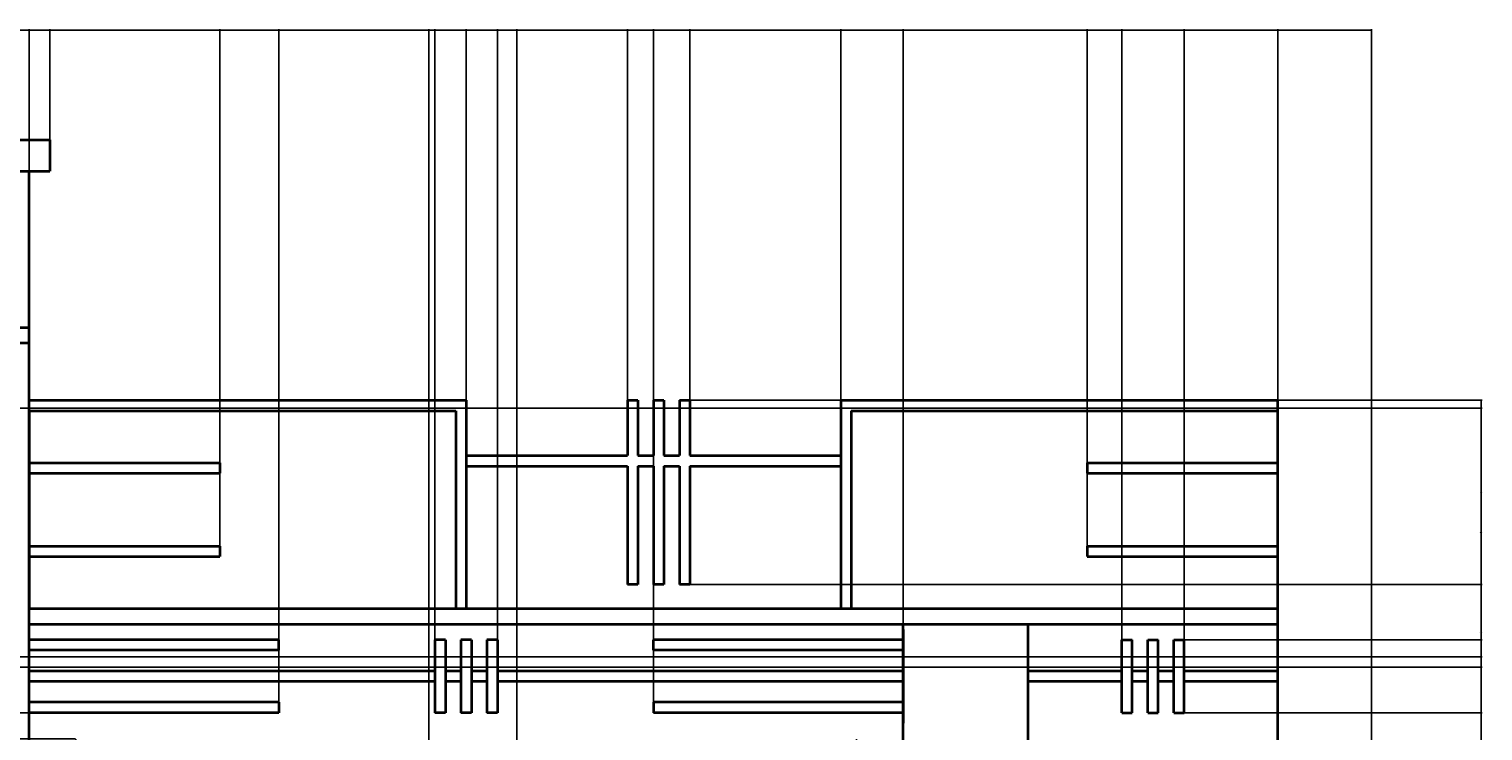
# Model space of a CAD drawing. Units: inches. Extents: x 2148 to 2587, y 1015 to 1466.
# Tile 7 of 7: x 2307 to 2586, y 1331 to 1466. Entities that reach past the tile are written whole.
import ezdxf

# ---------------------------------------------------------------- set-up
doc = ezdxf.new("R2010")
doc.units = ezdxf.units.IN
doc.layers.add('A-ANNO-DIMS', color=2, linetype='Continuous', lineweight=18)
doc.layers.add('A-ELEV', color=7, linetype='Continuous', lineweight=35)
doc.styles.get("Standard").update_dxf_attribs({"font": 'arial.ttf'})
doc.dimstyles.get("Standard").update_dxf_attribs({"dimtxt": 0.18, "dimasz": 0.18, "dimexe": 0.18, "dimexo": 0.0625, "dimgap": 0.09, "dimtad": 0, "dimtih": 1, "dimtoh": 1, "dimdec": 4, "dimzin": 0, "dimdsep": 46, "dimtxsty": 'Standard', "dimcen": 0.09, "dimadec": 0, "dimazin": 0, "dimtfac": 1, "dimtdec": 4, "dimtofl": 0, "dimtmove": 0, "dimatfit": 3, "dimfxl": 1, "dimtolj": 1, "dimtzin": 0, "dimarcsym": 0})

# ---------------------------------------------------------------- blocks, each defined once
blk = doc.blocks.new('*D8')
at = {"layer": 'A-ANNO-DIMS', "color": 0, "lineweight": -2, "transparency": 16777216}
for p, q in [((2183.03, 1444.81), (2183.03, 1466.02)), ((2183.21, 1465.84), (2246.75, 1465.84)), ((2310.85, 1465.84), (2247.31, 1465.84)), ((2311.03, 1444.81), (2311.03, 1466.02))]:
    blk.add_line(p, q, dxfattribs=at)
at = {"layer": 'A-ANNO-DIMS', "color": 0, "transparency": 16777216}
for points in [[(2183.21, 1465.87), (2183.21, 1465.81), (2183.03, 1465.84)], [(2310.85, 1465.87), (2310.85, 1465.81), (2311.03, 1465.84)]]:
    blk.add_solid(points, dxfattribs=at)
at = {"layer": 'Defpoints', "color": 0, "transparency": 16777216}
for p in [(2311.03, 1465.84), (2183.03, 1444.74), (2311.03, 1444.74)]:
    blk.add_point(p, dxfattribs=at)
at = {"layer": 'A-ANNO-DIMS', "color": 0, "transparency": 16777216, "insert": (2247.03, 1465.84), "char_height": 0.18, "attachment_point": 5}
blk.add_mtext('\\A1;128', dxfattribs=at)
blk = doc.blocks.new('*D9')
at = {"layer": 'A-ANNO-DIMS', "color": 0, "lineweight": -2, "transparency": 16777216}
for p, q in [((2311.03, 1444.81), (2311.03, 1466.02)), ((2311.21, 1465.84), (2437.74, 1465.84)), ((2564.85, 1465.84), (2438.32, 1465.84)), ((2565.03, 1305.54), (2565.03, 1466.02))]:
    blk.add_line(p, q, dxfattribs=at)
at = {"layer": 'A-ANNO-DIMS', "color": 0, "transparency": 16777216}
for points in [[(2311.21, 1465.87), (2311.21, 1465.81), (2311.03, 1465.84)], [(2564.85, 1465.87), (2564.85, 1465.81), (2565.03, 1465.84)]]:
    blk.add_solid(points, dxfattribs=at)
at = {"layer": 'Defpoints', "color": 0, "transparency": 16777216}
for p in [(2565.03, 1465.84), (2311.03, 1444.74), (2565.03, 1305.47)]:
    blk.add_point(p, dxfattribs=at)
at = {"layer": 'A-ANNO-DIMS', "color": 0, "transparency": 16777216, "insert": (2438.03, 1465.84), "char_height": 0.18, "attachment_point": 5}
blk.add_mtext('\\A1;254', dxfattribs=at)
blk = doc.blocks.new('*D32')
at = {"layer": 'A-ANNO-DIMS', "color": 0, "lineweight": -2, "transparency": 16777216}
for p, q in [((2547.1, 1394.74), (2586.31, 1394.74)), ((2586.13, 1394.56), (2586.13, 1350.29)), ((2586.13, 1305.65), (2586.13, 1349.93)), ((2565.1, 1305.47), (2586.31, 1305.47))]:
    blk.add_line(p, q, dxfattribs=at)
at = {"layer": 'A-ANNO-DIMS', "color": 0, "transparency": 16777216}
for points in [[(2586.1, 1394.56), (2586.16, 1394.56), (2586.13, 1394.74)], [(2586.1, 1305.65), (2586.16, 1305.65), (2586.13, 1305.47)]]:
    blk.add_solid(points, dxfattribs=at)
at = {"layer": 'Defpoints', "color": 0, "transparency": 16777216}
for p in [(2547.03, 1394.74), (2586.13, 1394.74), (2565.03, 1305.47)]:
    blk.add_point(p, dxfattribs=at)
at = {"layer": 'A-ANNO-DIMS', "color": 0, "transparency": 16777216, "insert": (2586.13, 1350.11), "char_height": 0.18, "attachment_point": 5}
blk.add_mtext('\\A1;89.27', dxfattribs=at)
blk = doc.blocks.new('*D33')
at = {"layer": 'A-ANNO-DIMS', "color": 0, "lineweight": -2, "transparency": 16777216}
for p, q in [((2307.03, 1394.81), (2307.03, 1466.02)), ((2307.21, 1465.84), (2324.89, 1465.84)), ((2343.5, 1465.84), (2325.82, 1465.84)), ((2343.68, 1366.81), (2343.68, 1466.02))]:
    blk.add_line(p, q, dxfattribs=at)
at = {"layer": 'A-ANNO-DIMS', "color": 0, "transparency": 16777216}
for points in [[(2307.21, 1465.87), (2307.21, 1465.81), (2307.03, 1465.84)], [(2343.5, 1465.87), (2343.5, 1465.81), (2343.68, 1465.84)]]:
    blk.add_solid(points, dxfattribs=at)
at = {"layer": 'Defpoints', "color": 0, "transparency": 16777216}
for p in [(2343.68, 1465.84), (2307.03, 1394.74), (2343.68, 1366.74)]:
    blk.add_point(p, dxfattribs=at)
at = {"layer": 'A-ANNO-DIMS', "color": 0, "transparency": 16777216, "insert": (2325.36, 1465.84), "char_height": 0.18, "attachment_point": 5}
blk.add_mtext('\\A1;36.645', dxfattribs=at)
blk = doc.blocks.new('*D34')
at = {"layer": 'A-ANNO-DIMS', "color": 0, "lineweight": -2, "transparency": 16777216}
for p, q in [((2343.68, 1366.81), (2343.68, 1466.02)), ((2343.86, 1465.84), (2348.9, 1465.84)), ((2354.85, 1465.84), (2349.81, 1465.84)), ((2355.03, 1334.81), (2355.03, 1466.02))]:
    blk.add_line(p, q, dxfattribs=at)
at = {"layer": 'A-ANNO-DIMS', "color": 0, "transparency": 16777216}
for points in [[(2343.86, 1465.87), (2343.86, 1465.81), (2343.68, 1465.84)], [(2354.85, 1465.87), (2354.85, 1465.81), (2355.03, 1465.84)]]:
    blk.add_solid(points, dxfattribs=at)
at = {"layer": 'Defpoints', "color": 0, "transparency": 16777216}
for p in [(2355.03, 1465.84), (2343.68, 1366.74), (2355.03, 1334.74)]:
    blk.add_point(p, dxfattribs=at)
at = {"layer": 'A-ANNO-DIMS', "color": 0, "transparency": 16777216, "insert": (2349.36, 1465.84), "char_height": 0.18, "attachment_point": 5}
blk.add_mtext('\\A1;11.355', dxfattribs=at)
blk = doc.blocks.new('*D35')
at = {"layer": 'A-ANNO-DIMS', "color": 0, "lineweight": -2, "transparency": 16777216}
for p, q in [((2355.03, 1334.81), (2355.03, 1466.02)), ((2355.21, 1465.84), (2369.82, 1465.84)), ((2384.85, 1465.84), (2370.25, 1465.84)), ((2385.03, 1334.81), (2385.03, 1466.02))]:
    blk.add_line(p, q, dxfattribs=at)
at = {"layer": 'A-ANNO-DIMS', "color": 0, "transparency": 16777216}
for points in [[(2355.21, 1465.87), (2355.21, 1465.81), (2355.03, 1465.84)], [(2384.85, 1465.87), (2384.85, 1465.81), (2385.03, 1465.84)]]:
    blk.add_solid(points, dxfattribs=at)
at = {"layer": 'Defpoints', "color": 0, "transparency": 16777216}
for p in [(2385.03, 1465.84), (2355.03, 1334.74), (2385.03, 1334.74)]:
    blk.add_point(p, dxfattribs=at)
at = {"layer": 'A-ANNO-DIMS', "color": 0, "transparency": 16777216, "insert": (2370.03, 1465.84), "char_height": 0.18, "attachment_point": 5}
blk.add_mtext('\\A1;30', dxfattribs=at)
blk = doc.blocks.new('*D36')
at = {"layer": 'A-ANNO-DIMS', "color": 0, "lineweight": -2, "transparency": 16777216}
for p, q in [((2385.03, 1334.81), (2385.03, 1466.02)), ((2385.21, 1465.84), (2387.88, 1465.84)), ((2390.85, 1465.84), (2388.18, 1465.84)), ((2391.03, 1394.81), (2391.03, 1466.02))]:
    blk.add_line(p, q, dxfattribs=at)
at = {"layer": 'A-ANNO-DIMS', "color": 0, "transparency": 16777216}
for points in [[(2385.21, 1465.87), (2385.21, 1465.81), (2385.03, 1465.84)], [(2390.85, 1465.87), (2390.85, 1465.81), (2391.03, 1465.84)]]:
    blk.add_solid(points, dxfattribs=at)
at = {"layer": 'Defpoints', "color": 0, "transparency": 16777216}
for p in [(2391.03, 1465.84), (2391.03, 1394.74), (2385.03, 1334.74)]:
    blk.add_point(p, dxfattribs=at)
at = {"layer": 'A-ANNO-DIMS', "color": 0, "transparency": 16777216, "insert": (2388.03, 1465.84), "char_height": 0.18, "attachment_point": 5}
blk.add_mtext('\\A1;6', dxfattribs=at)
blk = doc.blocks.new('*D37')
at = {"layer": 'A-ANNO-DIMS', "color": 0, "lineweight": -2, "transparency": 16777216}
for p, q in [((2391.03, 1394.81), (2391.03, 1466.02)), ((2391.21, 1465.84), (2393.88, 1465.84)), ((2396.85, 1465.84), (2394.18, 1465.84)), ((2397.03, 1334.81), (2397.03, 1466.02))]:
    blk.add_line(p, q, dxfattribs=at)
at = {"layer": 'A-ANNO-DIMS', "color": 0, "transparency": 16777216}
for points in [[(2391.21, 1465.87), (2391.21, 1465.81), (2391.03, 1465.84)], [(2396.85, 1465.87), (2396.85, 1465.81), (2397.03, 1465.84)]]:
    blk.add_solid(points, dxfattribs=at)
at = {"layer": 'Defpoints', "color": 0, "transparency": 16777216}
for p in [(2397.03, 1465.84), (2391.03, 1394.74), (2397.03, 1334.74)]:
    blk.add_point(p, dxfattribs=at)
at = {"layer": 'A-ANNO-DIMS', "color": 0, "transparency": 16777216, "insert": (2394.03, 1465.84), "char_height": 0.18, "attachment_point": 5}
blk.add_mtext('\\A1;6', dxfattribs=at)
blk = doc.blocks.new('*D38')
at = {"layer": 'A-ANNO-DIMS', "color": 0, "lineweight": -2, "transparency": 16777216}
for p, q in [((2397.03, 1334.81), (2397.03, 1466.02)), ((2397.21, 1465.84), (2409.31, 1465.84)), ((2421.85, 1465.84), (2409.76, 1465.84)), ((2422.03, 1394.81), (2422.03, 1466.02))]:
    blk.add_line(p, q, dxfattribs=at)
at = {"layer": 'A-ANNO-DIMS', "color": 0, "transparency": 16777216}
for points in [[(2397.21, 1465.87), (2397.21, 1465.81), (2397.03, 1465.84)], [(2421.85, 1465.87), (2421.85, 1465.81), (2422.03, 1465.84)]]:
    blk.add_solid(points, dxfattribs=at)
at = {"layer": 'Defpoints', "color": 0, "transparency": 16777216}
for p in [(2422.03, 1465.84), (2422.03, 1394.74), (2397.03, 1334.74)]:
    blk.add_point(p, dxfattribs=at)
at = {"layer": 'A-ANNO-DIMS', "color": 0, "transparency": 16777216, "insert": (2409.53, 1465.84), "char_height": 0.18, "attachment_point": 5}
blk.add_mtext('\\A1;25', dxfattribs=at)
blk = doc.blocks.new('*D39')
at = {"layer": 'A-ANNO-DIMS', "color": 0, "lineweight": -2, "transparency": 16777216}
for p, q in [((2422.03, 1394.81), (2422.03, 1466.02)), ((2422.21, 1465.84), (2424.38, 1465.84)), ((2426.85, 1465.84), (2424.68, 1465.84)), ((2427.03, 1334.81), (2427.03, 1466.02))]:
    blk.add_line(p, q, dxfattribs=at)
at = {"layer": 'A-ANNO-DIMS', "color": 0, "transparency": 16777216}
for points in [[(2422.21, 1465.87), (2422.21, 1465.81), (2422.03, 1465.84)], [(2426.85, 1465.87), (2426.85, 1465.81), (2427.03, 1465.84)]]:
    blk.add_solid(points, dxfattribs=at)
at = {"layer": 'Defpoints', "color": 0, "transparency": 16777216}
for p in [(2427.03, 1465.84), (2422.03, 1394.74), (2427.03, 1334.74)]:
    blk.add_point(p, dxfattribs=at)
at = {"layer": 'A-ANNO-DIMS', "color": 0, "transparency": 16777216, "insert": (2424.53, 1465.84), "char_height": 0.18, "attachment_point": 5}
blk.add_mtext('\\A1;5', dxfattribs=at)
blk = doc.blocks.new('*D40')
at = {"layer": 'A-ANNO-DIMS', "color": 0, "lineweight": -2, "transparency": 16777216}
for p, q in [((2427.03, 1334.81), (2427.03, 1466.02)), ((2427.21, 1465.84), (2430.39, 1465.84)), ((2433.85, 1465.84), (2430.68, 1465.84)), ((2434.03, 1394.81), (2434.03, 1466.02))]:
    blk.add_line(p, q, dxfattribs=at)
at = {"layer": 'A-ANNO-DIMS', "color": 0, "transparency": 16777216}
for points in [[(2427.21, 1465.87), (2427.21, 1465.81), (2427.03, 1465.84)], [(2433.85, 1465.87), (2433.85, 1465.81), (2434.03, 1465.84)]]:
    blk.add_solid(points, dxfattribs=at)
at = {"layer": 'Defpoints', "color": 0, "transparency": 16777216}
for p in [(2434.03, 1465.84), (2434.03, 1394.74), (2427.03, 1334.74)]:
    blk.add_point(p, dxfattribs=at)
at = {"layer": 'A-ANNO-DIMS', "color": 0, "transparency": 16777216, "insert": (2430.53, 1465.84), "char_height": 0.18, "attachment_point": 5}
blk.add_mtext('\\A1;7', dxfattribs=at)
blk = doc.blocks.new('*D41')
at = {"layer": 'A-ANNO-DIMS', "color": 0, "lineweight": -2, "transparency": 16777216}
for p, q in [((2434.03, 1394.81), (2434.03, 1466.02)), ((2434.21, 1465.84), (2448.31, 1465.84)), ((2462.85, 1465.84), (2448.75, 1465.84)), ((2463.03, 1394.81), (2463.03, 1466.02))]:
    blk.add_line(p, q, dxfattribs=at)
at = {"layer": 'A-ANNO-DIMS', "color": 0, "transparency": 16777216}
for points in [[(2434.21, 1465.87), (2434.21, 1465.81), (2434.03, 1465.84)], [(2462.85, 1465.87), (2462.85, 1465.81), (2463.03, 1465.84)]]:
    blk.add_solid(points, dxfattribs=at)
at = {"layer": 'Defpoints', "color": 0, "transparency": 16777216}
for p in [(2463.03, 1465.84), (2434.03, 1394.74), (2463.03, 1394.74)]:
    blk.add_point(p, dxfattribs=at)
at = {"layer": 'A-ANNO-DIMS', "color": 0, "transparency": 16777216, "insert": (2448.53, 1465.84), "char_height": 0.18, "attachment_point": 5}
blk.add_mtext('\\A1;29', dxfattribs=at)
blk = doc.blocks.new('*D42')
at = {"layer": 'A-ANNO-DIMS', "color": 0, "lineweight": -2, "transparency": 16777216}
for p, q in [((2463.03, 1394.81), (2463.03, 1466.02)), ((2463.21, 1465.84), (2468.82, 1465.84)), ((2474.85, 1465.84), (2469.24, 1465.84)), ((2475.03, 1351.81), (2475.03, 1466.02))]:
    blk.add_line(p, q, dxfattribs=at)
at = {"layer": 'A-ANNO-DIMS', "color": 0, "transparency": 16777216}
for points in [[(2463.21, 1465.87), (2463.21, 1465.81), (2463.03, 1465.84)], [(2474.85, 1465.87), (2474.85, 1465.81), (2475.03, 1465.84)]]:
    blk.add_solid(points, dxfattribs=at)
at = {"layer": 'Defpoints', "color": 0, "transparency": 16777216}
for p in [(2475.03, 1465.84), (2463.03, 1394.74), (2475.03, 1351.74)]:
    blk.add_point(p, dxfattribs=at)
at = {"layer": 'A-ANNO-DIMS', "color": 0, "transparency": 16777216, "insert": (2469.03, 1465.84), "char_height": 0.18, "attachment_point": 5}
blk.add_mtext('\\A1;12', dxfattribs=at)
blk = doc.blocks.new('*D43')
at = {"layer": 'A-ANNO-DIMS', "color": 0, "lineweight": -2, "transparency": 16777216}
for p, q in [((2475.03, 1351.81), (2475.03, 1466.02)), ((2475.21, 1465.84), (2492.25, 1465.84)), ((2510.21, 1465.84), (2493.18, 1465.84)), ((2510.39, 1366.81), (2510.39, 1466.02))]:
    blk.add_line(p, q, dxfattribs=at)
at = {"layer": 'A-ANNO-DIMS', "color": 0, "transparency": 16777216}
for points in [[(2475.21, 1465.87), (2475.21, 1465.81), (2475.03, 1465.84)], [(2510.21, 1465.87), (2510.21, 1465.81), (2510.39, 1465.84)]]:
    blk.add_solid(points, dxfattribs=at)
at = {"layer": 'Defpoints', "color": 0, "transparency": 16777216}
for p in [(2510.39, 1465.84), (2510.39, 1366.74), (2475.03, 1351.74)]:
    blk.add_point(p, dxfattribs=at)
at = {"layer": 'A-ANNO-DIMS', "color": 0, "transparency": 16777216, "insert": (2492.71, 1465.84), "char_height": 0.18, "attachment_point": 5}
blk.add_mtext('\\A1;35.355', dxfattribs=at)
blk = doc.blocks.new('*D44')
at = {"layer": 'A-ANNO-DIMS', "color": 0, "lineweight": -2, "transparency": 16777216}
for p, q in [((2510.39, 1366.81), (2510.39, 1466.02)), ((2510.57, 1465.84), (2513.32, 1465.84)), ((2516.85, 1465.84), (2514.11, 1465.84)), ((2517.03, 1334.81), (2517.03, 1466.02))]:
    blk.add_line(p, q, dxfattribs=at)
at = {"layer": 'A-ANNO-DIMS', "color": 0, "transparency": 16777216}
for points in [[(2510.57, 1465.87), (2510.57, 1465.81), (2510.39, 1465.84)], [(2516.85, 1465.87), (2516.85, 1465.81), (2517.03, 1465.84)]]:
    blk.add_solid(points, dxfattribs=at)
at = {"layer": 'Defpoints', "color": 0, "transparency": 16777216}
for p in [(2517.03, 1465.84), (2510.39, 1366.74), (2517.03, 1334.74)]:
    blk.add_point(p, dxfattribs=at)
at = {"layer": 'A-ANNO-DIMS', "color": 0, "transparency": 16777216, "insert": (2513.71, 1465.84), "char_height": 0.18, "attachment_point": 5}
blk.add_mtext('\\A1;6.645', dxfattribs=at)
blk = doc.blocks.new('*D45')
at = {"layer": 'A-ANNO-DIMS', "color": 0, "lineweight": -2, "transparency": 16777216}
for p, q in [((2517.03, 1334.81), (2517.03, 1466.02)), ((2517.21, 1465.84), (2522.82, 1465.84)), ((2528.85, 1465.84), (2523.24, 1465.84)), ((2529.03, 1334.81), (2529.03, 1466.02))]:
    blk.add_line(p, q, dxfattribs=at)
at = {"layer": 'A-ANNO-DIMS', "color": 0, "transparency": 16777216}
for points in [[(2517.21, 1465.87), (2517.21, 1465.81), (2517.03, 1465.84)], [(2528.85, 1465.87), (2528.85, 1465.81), (2529.03, 1465.84)]]:
    blk.add_solid(points, dxfattribs=at)
at = {"layer": 'Defpoints', "color": 0, "transparency": 16777216}
for p in [(2529.03, 1465.84), (2517.03, 1334.74), (2529.03, 1334.74)]:
    blk.add_point(p, dxfattribs=at)
at = {"layer": 'A-ANNO-DIMS', "color": 0, "transparency": 16777216, "insert": (2523.03, 1465.84), "char_height": 0.18, "attachment_point": 5}
blk.add_mtext('\\A1;12', dxfattribs=at)
blk = doc.blocks.new('*D46')
at = {"layer": 'A-ANNO-DIMS', "color": 0, "lineweight": -2, "transparency": 16777216}
for p, q in [((2529.03, 1334.81), (2529.03, 1466.02)), ((2529.21, 1465.84), (2537.82, 1465.84)), ((2546.85, 1465.84), (2538.24, 1465.84)), ((2547.03, 1394.81), (2547.03, 1466.02))]:
    blk.add_line(p, q, dxfattribs=at)
at = {"layer": 'A-ANNO-DIMS', "color": 0, "transparency": 16777216}
for points in [[(2529.21, 1465.87), (2529.21, 1465.81), (2529.03, 1465.84)], [(2546.85, 1465.87), (2546.85, 1465.81), (2547.03, 1465.84)]]:
    blk.add_solid(points, dxfattribs=at)
at = {"layer": 'Defpoints', "color": 0, "transparency": 16777216}
for p in [(2547.03, 1465.84), (2547.03, 1394.74), (2529.03, 1334.74)]:
    blk.add_point(p, dxfattribs=at)
at = {"layer": 'A-ANNO-DIMS', "color": 0, "transparency": 16777216, "insert": (2538.03, 1465.84), "char_height": 0.18, "attachment_point": 5}
blk.add_mtext('\\A1;18', dxfattribs=at)
blk = doc.blocks.new('*D47')
at = {"layer": 'A-ANNO-DIMS', "color": 0, "lineweight": -2, "transparency": 16777216}
for p, q in [((2307.03, 1334.68), (2307.03, 1015.46)), ((2316.03, 1329.68), (2316.03, 1015.46)), ((2307.21, 1015.64), (2311.39, 1015.64)), ((2315.85, 1015.64), (2311.68, 1015.64))]:
    blk.add_line(p, q, dxfattribs=at)
at = {"layer": 'A-ANNO-DIMS', "color": 0, "transparency": 16777216}
for points in [[(2307.21, 1015.67), (2307.21, 1015.61), (2307.03, 1015.64)], [(2315.85, 1015.67), (2315.85, 1015.61), (2316.03, 1015.64)]]:
    blk.add_solid(points, dxfattribs=at)
at = {"layer": 'Defpoints', "color": 0, "transparency": 16777216}
for p in [(2307.03, 1334.74), (2316.03, 1329.74), (2316.03, 1015.64)]:
    blk.add_point(p, dxfattribs=at)
at = {"layer": 'A-ANNO-DIMS', "color": 0, "transparency": 16777216, "insert": (2311.53, 1015.64), "char_height": 0.18, "attachment_point": 5}
blk.add_mtext('\\A1;9', dxfattribs=at)
blk = doc.blocks.new('*D53')
at = {"layer": 'A-ANNO-DIMS', "color": 0, "lineweight": -2, "transparency": 16777216}
for p, q in [((2475.03, 1351.68), (2475.03, 1015.46)), ((2466.03, 1329.68), (2466.03, 1015.46)), ((2466.21, 1015.64), (2470.39, 1015.64)), ((2474.85, 1015.64), (2470.68, 1015.64))]:
    blk.add_line(p, q, dxfattribs=at)
at = {"layer": 'A-ANNO-DIMS', "color": 0, "transparency": 16777216}
for points in [[(2466.21, 1015.67), (2466.21, 1015.61), (2466.03, 1015.64)], [(2474.85, 1015.67), (2474.85, 1015.61), (2475.03, 1015.64)]]:
    blk.add_solid(points, dxfattribs=at)
at = {"layer": 'Defpoints', "color": 0, "transparency": 16777216}
for p in [(2475.03, 1351.74), (2466.03, 1329.74), (2475.03, 1015.64)]:
    blk.add_point(p, dxfattribs=at)
at = {"layer": 'A-ANNO-DIMS', "color": 0, "transparency": 16777216, "insert": (2470.53, 1015.64), "char_height": 0.18, "attachment_point": 5}
blk.add_mtext('\\A1;9', dxfattribs=at)
blk = doc.blocks.new('*D54')
at = {"layer": 'A-ANNO-DIMS', "color": 0, "lineweight": -2, "transparency": 16777216}
for p, q in [((2475.03, 1351.68), (2475.03, 1015.46)), ((2499.03, 1329.68), (2499.03, 1015.46)), ((2475.21, 1015.64), (2486.81, 1015.64)), ((2498.85, 1015.64), (2487.25, 1015.64))]:
    blk.add_line(p, q, dxfattribs=at)
at = {"layer": 'A-ANNO-DIMS', "color": 0, "transparency": 16777216}
for points in [[(2475.21, 1015.67), (2475.21, 1015.61), (2475.03, 1015.64)], [(2498.85, 1015.67), (2498.85, 1015.61), (2499.03, 1015.64)]]:
    blk.add_solid(points, dxfattribs=at)
at = {"layer": 'Defpoints', "color": 0, "transparency": 16777216}
for p in [(2475.03, 1351.74), (2499.03, 1329.74), (2499.03, 1015.64)]:
    blk.add_point(p, dxfattribs=at)
at = {"layer": 'A-ANNO-DIMS', "color": 0, "transparency": 16777216, "insert": (2487.03, 1015.64), "char_height": 0.18, "attachment_point": 5}
blk.add_mtext('\\A1;24', dxfattribs=at)
blk = doc.blocks.new('*D63')
at = {"layer": 'A-ANNO-DIMS', "color": 0, "lineweight": -2, "transparency": 16777216}
for p, q in [((2306.97, 1334.74), (2147.75, 1334.74)), ((2147.93, 1334.56), (2147.93, 1332.42)), ((2147.93, 1329.92), (2147.93, 1332.06)), ((2315.97, 1329.74), (2147.75, 1329.74))]:
    blk.add_line(p, q, dxfattribs=at)
at = {"layer": 'A-ANNO-DIMS', "color": 0, "transparency": 16777216}
for points in [[(2147.9, 1334.56), (2147.96, 1334.56), (2147.93, 1334.74)], [(2147.9, 1329.92), (2147.96, 1329.92), (2147.93, 1329.74)]]:
    blk.add_solid(points, dxfattribs=at)
at = {"layer": 'Defpoints', "color": 0, "transparency": 16777216}
for p in [(2147.93, 1334.74), (2307.03, 1334.74), (2316.03, 1329.74)]:
    blk.add_point(p, dxfattribs=at)
at = {"layer": 'A-ANNO-DIMS', "color": 0, "transparency": 16777216, "insert": (2147.93, 1332.24), "char_height": 0.18, "attachment_point": 5}
blk.add_mtext('\\A1;5', dxfattribs=at)
blk = doc.blocks.new('*D71')
at = {"layer": 'A-ANNO-DIMS', "color": 0, "lineweight": -2, "transparency": 16777216}
for p, q in [((2529.1, 1348.74), (2586.31, 1348.74)), ((2586.13, 1348.56), (2586.13, 1341.92)), ((2586.13, 1334.92), (2586.13, 1341.56)), ((2529.1, 1334.74), (2586.31, 1334.74))]:
    blk.add_line(p, q, dxfattribs=at)
at = {"layer": 'A-ANNO-DIMS', "color": 0, "transparency": 16777216}
for points in [[(2586.1, 1348.56), (2586.16, 1348.56), (2586.13, 1348.74)], [(2586.1, 1334.92), (2586.16, 1334.92), (2586.13, 1334.74)]]:
    blk.add_solid(points, dxfattribs=at)
at = {"layer": 'Defpoints', "color": 0, "transparency": 16777216}
for p in [(2529.03, 1348.74), (2586.13, 1348.74), (2529.03, 1334.74)]:
    blk.add_point(p, dxfattribs=at)
at = {"layer": 'A-ANNO-DIMS', "color": 0, "transparency": 16777216, "insert": (2586.13, 1341.74), "char_height": 0.18, "attachment_point": 5}
blk.add_mtext('\\A1;14', dxfattribs=at)
blk = doc.blocks.new('*D72')
at = {"layer": 'A-ANNO-DIMS', "color": 0, "lineweight": -2, "transparency": 16777216}
for p, q in [((2434.1, 1394.74), (2586.31, 1394.74)), ((2586.13, 1394.56), (2586.13, 1377.24)), ((2586.13, 1359.56), (2586.13, 1376.88)), ((2434.1, 1359.38), (2586.31, 1359.38))]:
    blk.add_line(p, q, dxfattribs=at)
at = {"layer": 'A-ANNO-DIMS', "color": 0, "transparency": 16777216}
for points in [[(2586.1, 1394.56), (2586.16, 1394.56), (2586.13, 1394.74)], [(2586.1, 1359.56), (2586.16, 1359.56), (2586.13, 1359.38)]]:
    blk.add_solid(points, dxfattribs=at)
at = {"layer": 'Defpoints', "color": 0, "transparency": 16777216}
for p in [(2434.03, 1394.74), (2586.13, 1394.74), (2434.03, 1359.38)]:
    blk.add_point(p, dxfattribs=at)
at = {"layer": 'A-ANNO-DIMS', "color": 0, "transparency": 16777216, "insert": (2586.13, 1377.06), "char_height": 0.18, "attachment_point": 5}
blk.add_mtext('\\A1;35.37', dxfattribs=at)
blk = doc.blocks.new('*D95')
at = {"layer": 'A-ANNO-DIMS', "color": 0, "lineweight": -2, "transparency": 16777216}
for p, q in [((2260.35, 1343.49), (2586.31, 1343.49)), ((2586.13, 1343.31), (2586.13, 1295.67)), ((2586.13, 1247.67), (2586.13, 1295.31)), ((2260.35, 1247.49), (2586.31, 1247.49))]:
    blk.add_line(p, q, dxfattribs=at)
at = {"layer": 'A-ANNO-DIMS', "color": 0, "transparency": 16777216}
for points in [[(2586.1, 1343.31), (2586.16, 1343.31), (2586.13, 1343.49)], [(2586.1, 1247.67), (2586.16, 1247.67), (2586.13, 1247.49)]]:
    blk.add_solid(points, dxfattribs=at)
at = {"layer": 'Defpoints', "color": 0, "transparency": 16777216}
for p in [(2260.29, 1343.49), (2586.13, 1343.49), (2260.29, 1247.49)]:
    blk.add_point(p, dxfattribs=at)
at = {"layer": 'A-ANNO-DIMS', "color": 0, "transparency": 16777216, "insert": (2586.13, 1295.49), "char_height": 0.18, "attachment_point": 5}
blk.add_mtext('\\A1;96', dxfattribs=at)
blk = doc.blocks.new('*D96')
at = {"layer": 'A-ANNO-DIMS', "color": 0, "lineweight": -2, "transparency": 16777216}
for p, q in [((2260.35, 1345.49), (2586.31, 1345.49)), ((2586.13, 1345.31), (2586.13, 1344.67)), ((2586.13, 1343.67), (2586.13, 1344.31)), ((2260.35, 1343.49), (2586.31, 1343.49))]:
    blk.add_line(p, q, dxfattribs=at)
at = {"layer": 'A-ANNO-DIMS', "color": 0, "transparency": 16777216}
for points in [[(2586.1, 1345.31), (2586.16, 1345.31), (2586.13, 1345.49)], [(2586.1, 1343.67), (2586.16, 1343.67), (2586.13, 1343.49)]]:
    blk.add_solid(points, dxfattribs=at)
at = {"layer": 'Defpoints', "color": 0, "transparency": 16777216}
for p in [(2260.29, 1345.49), (2586.13, 1345.49), (2260.29, 1343.49)]:
    blk.add_point(p, dxfattribs=at)
at = {"layer": 'A-ANNO-DIMS', "color": 0, "transparency": 16777216, "insert": (2586.13, 1344.49), "char_height": 0.18, "attachment_point": 5}
blk.add_mtext('\\A1;2', dxfattribs=at)
blk = doc.blocks.new('*D97')
at = {"layer": 'A-ANNO-DIMS', "color": 0, "lineweight": -2, "transparency": 16777216}
for p, q in [((2262.35, 1393.24), (2586.31, 1393.24)), ((2586.13, 1393.06), (2586.13, 1369.55)), ((2586.13, 1345.67), (2586.13, 1369.18)), ((2260.35, 1345.49), (2586.31, 1345.49))]:
    blk.add_line(p, q, dxfattribs=at)
at = {"layer": 'A-ANNO-DIMS', "color": 0, "transparency": 16777216}
for points in [[(2586.1, 1393.06), (2586.16, 1393.06), (2586.13, 1393.24)], [(2586.1, 1345.67), (2586.16, 1345.67), (2586.13, 1345.49)]]:
    blk.add_solid(points, dxfattribs=at)
at = {"layer": 'Defpoints', "color": 0, "transparency": 16777216}
for p in [(2262.29, 1393.24), (2586.13, 1393.24), (2260.29, 1345.49)]:
    blk.add_point(p, dxfattribs=at)
at = {"layer": 'A-ANNO-DIMS', "color": 0, "transparency": 16777216, "insert": (2586.13, 1369.36), "char_height": 0.18, "attachment_point": 5}
blk.add_mtext('\\A1;47.75', dxfattribs=at)
blk = doc.blocks.new('*D98')
at = {"layer": 'A-ANNO-DIMS', "color": 0, "lineweight": -2, "transparency": 16777216}
for p, q in [((2383.84, 1054.81), (2383.84, 1466.02)), ((2384.02, 1465.84), (2391.92, 1465.84)), ((2400.59, 1465.84), (2392.69, 1465.84)), ((2400.77, 1054.81), (2400.77, 1466.02))]:
    blk.add_line(p, q, dxfattribs=at)
at = {"layer": 'A-ANNO-DIMS', "color": 0, "transparency": 16777216}
for points in [[(2384.02, 1465.87), (2384.02, 1465.81), (2383.84, 1465.84)], [(2400.59, 1465.87), (2400.59, 1465.81), (2400.77, 1465.84)]]:
    blk.add_solid(points, dxfattribs=at)
at = {"layer": 'Defpoints', "color": 0, "transparency": 16777216}
for p in [(2400.77, 1465.84), (2383.84, 1054.74), (2400.77, 1054.74)]:
    blk.add_point(p, dxfattribs=at)
at = {"layer": 'A-ANNO-DIMS', "color": 0, "transparency": 16777216, "insert": (2392.3, 1465.84), "char_height": 0.18, "attachment_point": 5}
blk.add_mtext('\\A1;16.93', dxfattribs=at)

msp = doc.modelspace()

# ---------------------------------------------------------------- linework, layer by layer
at = {"layer": 'A-ELEV'}
for p, q in [((2183.0343, 1444.7427), (2311.0343, 1444.7427)), ((2311.0343, 1444.7427), (2311.0343, 1438.7427)), ((2183.0343, 1438.7427), (2311.0343, 1438.7427)), ((2307.0343, 1166.7427), (2307.0343, 1438.7427)), ((2187.0343, 1408.7427), (2307.0343, 1408.7427)), ((2283.0343, 1405.7427), (2307.0343, 1405.7427)), ((2307.0343, 1394.7427), (2391.0343, 1394.7427)), ((2391.0343, 1394.7427), (2391.0343, 1354.7427)), ((2422.0343, 1394.7427), (2422.0343, 1384.1057)), ((2422.0343, 1394.7427), (2424.0343, 1394.7427)), ((2424.0343, 1394.7427), (2424.0343, 1384.1057)), ((2427.0343, 1394.7427), (2427.0343, 1384.1057)), ((2427.0343, 1394.7427), (2429.0343, 1394.7427)), ((2429.0343, 1394.7427), (2429.0343, 1384.1057)), ((2432.0343, 1394.7427), (2432.0343, 1384.1057)), ((2432.0343, 1394.7427), (2434.0343, 1394.7427)), ((2434.0343, 1394.7427), (2434.0343, 1384.1057)), ((2463.0343, 1394.7427), (2463.0343, 1354.7427)), ((2463.0343, 1394.7427), (2547.0343, 1394.7427)), ((2547.0343, 1048.7427), (2547.0343, 1394.7427)), ((2307.0343, 1392.7427), (2389.0343, 1392.7427)), ((2307.0343, 1392.7427), (2307.0343, 1354.7427)), ((2389.0343, 1392.7427), (2389.0343, 1354.7427)), ((2465.0343, 1392.7427), (2547.0343, 1392.7427)), ((2465.0343, 1392.7427), (2465.0343, 1354.7427)), ((2391.0343, 1384.1057), (2422.0343, 1384.1057)), ((2424.0343, 1384.1057), (2427.0343, 1384.1057)), ((2429.0343, 1384.1057), (2432.0343, 1384.1057)), ((2434.0343, 1384.1057), (2463.0343, 1384.1057)), ((2307.0343, 1382.7427), (2343.6794, 1382.7427)), ((2307.0343, 1380.7427), (2343.6794, 1380.7427)), ((2343.6794, 1382.7427), (2343.6794, 1380.7427)), ((2391.0343, 1382.1057), (2422.0343, 1382.1057)), ((2422.0343, 1382.1057), (2422.0343, 1359.3759)), ((2424.0343, 1382.1057), (2424.0343, 1359.3759)), ((2424.0343, 1382.1057), (2427.0343, 1382.1057)), ((2427.0343, 1382.1057), (2427.0343, 1359.3759)), ((2429.0343, 1382.1057), (2432.0343, 1382.1057)), ((2429.0343, 1382.1057), (2429.0343, 1359.3759)), ((2432.0343, 1382.1057), (2432.0343, 1359.3759)), ((2434.0343, 1382.1057), (2463.0343, 1382.1057)), ((2434.0343, 1382.1057), (2434.0343, 1359.3759)), ((2510.3891, 1382.7427), (2547.0343, 1382.7427)), ((2510.3891, 1382.7427), (2510.3891, 1380.7427)), ((2510.3891, 1380.7427), (2547.0343, 1380.7427)), ((2307.0343, 1366.7427), (2343.6794, 1366.7427)), ((2343.6794, 1366.7427), (2343.6794, 1364.7427)), ((2510.3891, 1366.7427), (2547.0343, 1366.7427)), ((2510.3891, 1366.7427), (2510.3891, 1364.7427)), ((2307.0343, 1364.7427), (2343.6794, 1364.7427)), ((2510.3891, 1364.7427), (2547.0343, 1364.7427)), ((2424.0343, 1359.3759), (2422.0343, 1359.3759)), ((2429.0343, 1359.3759), (2427.0343, 1359.3759)), ((2434.0343, 1359.3759), (2432.0343, 1359.3759)), ((2307.0343, 1354.7427), (2547.0343, 1354.7427)), ((2307.0343, 1351.7427), (2547.0343, 1351.7427)), ((2475.0343, 1166.7427), (2475.0343, 1351.7427)), ((2475.0343, 1350.7427), (2475.0343, 1332.7427)), ((2499.0343, 1166.7427), (2499.0343, 1351.7427)), ((2355.0343, 1348.7427), (2307.0343, 1348.7427)), ((2355.0343, 1346.7427), (2307.0343, 1346.7427)), ((2355.0343, 1346.7427), (2355.0343, 1348.7427)), ((2385.0343, 1348.7427), (2385.0343, 1334.7427)), ((2387.0343, 1348.7427), (2385.0343, 1348.7427)), ((2387.0343, 1348.7427), (2387.0343, 1334.7427)), ((2390.0343, 1348.7427), (2390.0343, 1334.7427)), ((2392.0343, 1348.7427), (2390.0343, 1348.7427)), ((2392.0343, 1348.7427), (2392.0343, 1334.7427)), ((2395.0343, 1348.7427), (2395.0343, 1334.7427)), ((2397.0343, 1348.7427), (2395.0343, 1348.7427)), ((2397.0343, 1348.7427), (2397.0343, 1334.7427)), ((2475.0343, 1348.7427), (2427.0343, 1348.7427)), ((2427.0343, 1346.7427), (2427.0343, 1348.7427)), ((2475.0343, 1346.7427), (2427.0343, 1346.7427)), ((2517.0343, 1334.7427), (2517.0343, 1348.7427)), ((2517.0343, 1348.7427), (2519.0343, 1348.7427)), ((2519.0343, 1334.7427), (2519.0343, 1348.7427)), ((2522.0343, 1334.7427), (2522.0343, 1348.7427)), ((2522.0343, 1348.7427), (2524.0343, 1348.7427)), ((2524.0343, 1334.7427), (2524.0343, 1348.7427)), ((2527.0343, 1334.7427), (2527.0343, 1348.7427)), ((2527.0343, 1348.7427), (2529.0343, 1348.7427)), ((2529.0343, 1334.7427), (2529.0343, 1348.7427)), ((2385.0343, 1342.7427), (2307.0343, 1342.7427)), ((2390.0343, 1342.7427), (2387.0343, 1342.7427)), ((2395.0343, 1342.7427), (2392.0343, 1342.7427)), ((2475.0343, 1342.7427), (2397.0343, 1342.7427)), ((2517.0343, 1342.7427), (2499.0343, 1342.7427)), ((2522.0343, 1342.7427), (2519.0343, 1342.7427)), ((2522.0343, 1342.7427), (2519.0343, 1342.7427)), ((2527.0343, 1342.7427), (2524.0343, 1342.7427)), ((2527.0343, 1342.7427), (2524.0343, 1342.7427)), ((2547.0343, 1342.7427), (2529.0343, 1342.7427)), ((2385.0343, 1340.7427), (2307.0343, 1340.7427)), ((2390.0343, 1340.7427), (2387.0343, 1340.7427)), ((2395.0343, 1340.7427), (2392.0343, 1340.7427)), ((2475.0343, 1340.7427), (2397.0343, 1340.7427)), ((2517.0343, 1340.7427), (2499.0343, 1340.7427)), ((2522.0343, 1340.7427), (2519.0343, 1340.7427)), ((2522.0343, 1340.7427), (2519.0343, 1340.7427)), ((2527.0343, 1340.7427), (2524.0343, 1340.7427)), ((2527.0343, 1340.7427), (2524.0343, 1340.7427)), ((2547.0343, 1340.7427), (2529.0343, 1340.7427)), ((2355.0343, 1336.7427), (2307.0343, 1336.7427)), ((2355.0343, 1336.7427), (2355.0343, 1334.7427)), ((2475.0343, 1336.7427), (2427.0343, 1336.7427)), ((2427.0343, 1336.7427), (2427.0343, 1334.7427)), ((2355.0343, 1334.7427), (2307.0343, 1334.7427)), ((2387.0343, 1334.7427), (2385.0343, 1334.7427)), ((2392.0343, 1334.7427), (2390.0343, 1334.7427)), ((2397.0343, 1334.7427), (2395.0343, 1334.7427)), ((2475.0343, 1334.7427), (2427.0343, 1334.7427)), ((2517.0343, 1334.7427), (2519.0343, 1334.7427)), ((2522.0343, 1334.7427), (2524.0343, 1334.7427)), ((2527.0343, 1334.7427), (2529.0343, 1334.7427))]:
    msp.add_line(p, q, dxfattribs=at)

# ---------------------------------------------------------------- dimensions: what is measured, and where the dimension line sits
at = {"layer": 'A-ANNO-DIMS'}
for base, p1, p2, override, picture, middle in [((2311.0343, 1465.8427), (2183.0343, 1444.7427), (2311.0343, 1444.7427), {"dimdec": 0, "dimlfac": 1, "dimrnd": 0, "dimzin": 0, "dimdsep": 46, "dimlunit": 2}, '*D8', (2247.0343, 1465.8427)), ((2343.6794, 1465.8427), (2307.0343, 1394.7427), (2343.6794, 1366.7427), {"dimdec": 3, "dimlfac": 1, "dimrnd": 0, "dimzin": 0, "dimdsep": 46, "dimlunit": 2}, '*D33', (2325.3568, 1465.8427)), ((2565.0343, 1465.8427), (2311.0343, 1444.7427), (2565.0343, 1305.4734), {"dimdec": 0, "dimlfac": 1, "dimrnd": 0, "dimzin": 0, "dimdsep": 46, "dimlunit": 2}, '*D9', (2438.0343, 1465.8427)), ((2355.0343, 1465.8427), (2343.6794, 1366.7427), (2355.0343, 1334.7427), {"dimdec": 3, "dimlfac": 1, "dimrnd": 0, "dimzin": 0, "dimdsep": 46, "dimlunit": 2}, '*D34', (2349.3568, 1465.8427)), ((2385.0343, 1465.8427), (2355.0343, 1334.7427), (2385.0343, 1334.7427), {"dimdec": 0, "dimlfac": 1, "dimrnd": 0, "dimzin": 0, "dimdsep": 46, "dimlunit": 2}, '*D35', (2370.0343, 1465.8427)), ((2400.7695, 1465.8427), (2383.84, 1054.7427), (2400.7695, 1054.7427), {"dimdec": 2, "dimlfac": 1, "dimrnd": 0, "dimzin": 0, "dimdsep": 46, "dimlunit": 2}, '*D98', (2392.3048, 1465.8427)), ((2391.0343, 1465.8427), (2385.0343, 1334.7427), (2391.0343, 1394.7427), {"dimdec": 0, "dimlfac": 1, "dimrnd": 0, "dimzin": 0, "dimdsep": 46, "dimlunit": 2}, '*D36', (2388.0343, 1465.8427)), ((2397.0343, 1465.8427), (2391.0343, 1394.7427), (2397.0343, 1334.7427), {"dimdec": 0, "dimlfac": 1, "dimrnd": 0, "dimzin": 0, "dimdsep": 46, "dimlunit": 2}, '*D37', (2394.0343, 1465.8427)), ((2422.0343, 1465.8427), (2397.0343, 1334.7427), (2422.0343, 1394.7427), {"dimdec": 0, "dimlfac": 1, "dimrnd": 0, "dimzin": 0, "dimdsep": 46, "dimlunit": 2}, '*D38', (2409.5343, 1465.8427)), ((2427.0343, 1465.8427), (2422.0343, 1394.7427), (2427.0343, 1334.7427), {"dimdec": 0, "dimlfac": 1, "dimrnd": 0, "dimzin": 0, "dimdsep": 46, "dimlunit": 2}, '*D39', (2424.5343, 1465.8427)), ((2434.0343, 1465.8427), (2427.0343, 1334.7427), (2434.0343, 1394.7427), {"dimdec": 0, "dimlfac": 1, "dimrnd": 0, "dimzin": 0, "dimdsep": 46, "dimlunit": 2}, '*D40', (2430.5343, 1465.8427)), ((2463.0343, 1465.8427), (2434.0343, 1394.7427), (2463.0343, 1394.7427), {"dimdec": 0, "dimlfac": 1, "dimrnd": 0, "dimzin": 0, "dimdsep": 46, "dimlunit": 2}, '*D41', (2448.5343, 1465.8427)), ((2475.0343, 1465.8427), (2463.0343, 1394.7427), (2475.0343, 1351.7427), {"dimdec": 0, "dimlfac": 1, "dimrnd": 0, "dimzin": 0, "dimdsep": 46, "dimlunit": 2}, '*D42', (2469.0343, 1465.8427)), ((2510.3891, 1465.8427), (2475.0343, 1351.7427), (2510.3891, 1366.7427), {"dimdec": 3, "dimlfac": 1, "dimrnd": 0, "dimzin": 0, "dimdsep": 46, "dimlunit": 2}, '*D43', (2492.7117, 1465.8427)), ((2517.0343, 1465.8427), (2510.3891, 1366.7427), (2517.0343, 1334.7427), {"dimdec": 3, "dimlfac": 1, "dimrnd": 0, "dimzin": 0, "dimdsep": 46, "dimlunit": 2}, '*D44', (2513.7117, 1465.8427)), ((2529.0343, 1465.8427), (2517.0343, 1334.7427), (2529.0343, 1334.7427), {"dimdec": 0, "dimlfac": 1, "dimrnd": 0, "dimzin": 0, "dimdsep": 46, "dimlunit": 2}, '*D45', (2523.0343, 1465.8427)), ((2547.0343, 1465.8427), (2529.0343, 1334.7427), (2547.0343, 1394.7427), {"dimdec": 0, "dimlfac": 1, "dimrnd": 0, "dimzin": 0, "dimdsep": 46, "dimlunit": 2}, '*D46', (2538.0343, 1465.8427)), ((2475.0343, 1015.6427), (2466.0343, 1329.7427), (2475.0343, 1351.7427), {"dimdec": 0, "dimlfac": 1, "dimrnd": 0, "dimzin": 0, "dimdsep": 46, "dimlunit": 2}, '*D53', (2470.5343, 1015.6427)), ((2499.0343, 1015.6427), (2475.0343, 1351.7427), (2499.0343, 1329.7427), {"dimdec": 0, "dimlfac": 1, "dimrnd": 0, "dimzin": 0, "dimdsep": 46, "dimlunit": 2}, '*D54', (2487.0343, 1015.6427)), ((2316.0343, 1015.6427), (2307.0343, 1334.7427), (2316.0343, 1329.7427), {"dimdec": 0, "dimlfac": 1, "dimrnd": 0, "dimzin": 0, "dimdsep": 46, "dimlunit": 2}, '*D47', (2311.5343, 1015.6427))]:
    dim = msp.add_linear_dim(base=base, p1=p1, p2=p2, dimstyle='Standard', override=override, dxfattribs=at)
    dim.commit()
    dim.dimension.update_dxf_attribs({"geometry": picture, "text_midpoint": middle})
for base, p1, p2, override, picture, middle in [((2586.1343, 1394.7427), (2434.0343, 1359.3759), (2434.0343, 1394.7427), {"dimdec": 2, "dimlfac": 1, "dimrnd": 0, "dimzin": 0, "dimdsep": 46, "dimlunit": 2}, '*D72', (2586.1343, 1377.0593)), ((2586.1343, 1394.7427), (2565.0343, 1305.4734), (2547.0343, 1394.7427), {"dimdec": 2, "dimlfac": 1, "dimrnd": 0, "dimzin": 0, "dimdsep": 46, "dimlunit": 2}, '*D32', (2586.1343, 1350.1081)), ((2586.1343, 1393.2389), (2260.287, 1345.4885), (2262.287, 1393.2389), {"dimdec": 2, "dimlfac": 1, "dimrnd": 0, "dimzin": 0, "dimdsep": 46, "dimlunit": 2}, '*D97', (2586.1343, 1369.3637)), ((2586.1343, 1348.7427), (2529.0343, 1334.7427), (2529.0343, 1348.7427), {"dimdec": 0, "dimlfac": 1, "dimrnd": 0, "dimzin": 0, "dimdsep": 46, "dimlunit": 2}, '*D71', (2586.1343, 1341.7427)), ((2586.1343, 1345.4885), (2260.287, 1343.4885), (2260.287, 1345.4885), {"dimdec": 0, "dimlfac": 1, "dimrnd": 0, "dimzin": 0, "dimdsep": 46, "dimlunit": 2}, '*D96', (2586.1343, 1344.4885)), ((2586.1343, 1343.4885), (2260.287, 1247.4885), (2260.287, 1343.4885), {"dimdec": 0, "dimlfac": 1, "dimrnd": 0, "dimzin": 0, "dimdsep": 46, "dimlunit": 2}, '*D95', (2586.1343, 1295.4885)), ((2147.9343, 1334.7427), (2316.0343, 1329.7427), (2307.0343, 1334.7427), {"dimdec": 0, "dimlfac": 1, "dimrnd": 0, "dimzin": 0, "dimdsep": 46, "dimlunit": 2}, '*D63', (2147.9343, 1332.2427))]:
    dim = msp.add_linear_dim(base=base, p1=p1, p2=p2, angle=90, dimstyle='Standard', override=override, dxfattribs=at)
    dim.commit()
    dim.dimension.update_dxf_attribs({"geometry": picture, "text_midpoint": middle})

doc.saveas('drawing.dxf')
